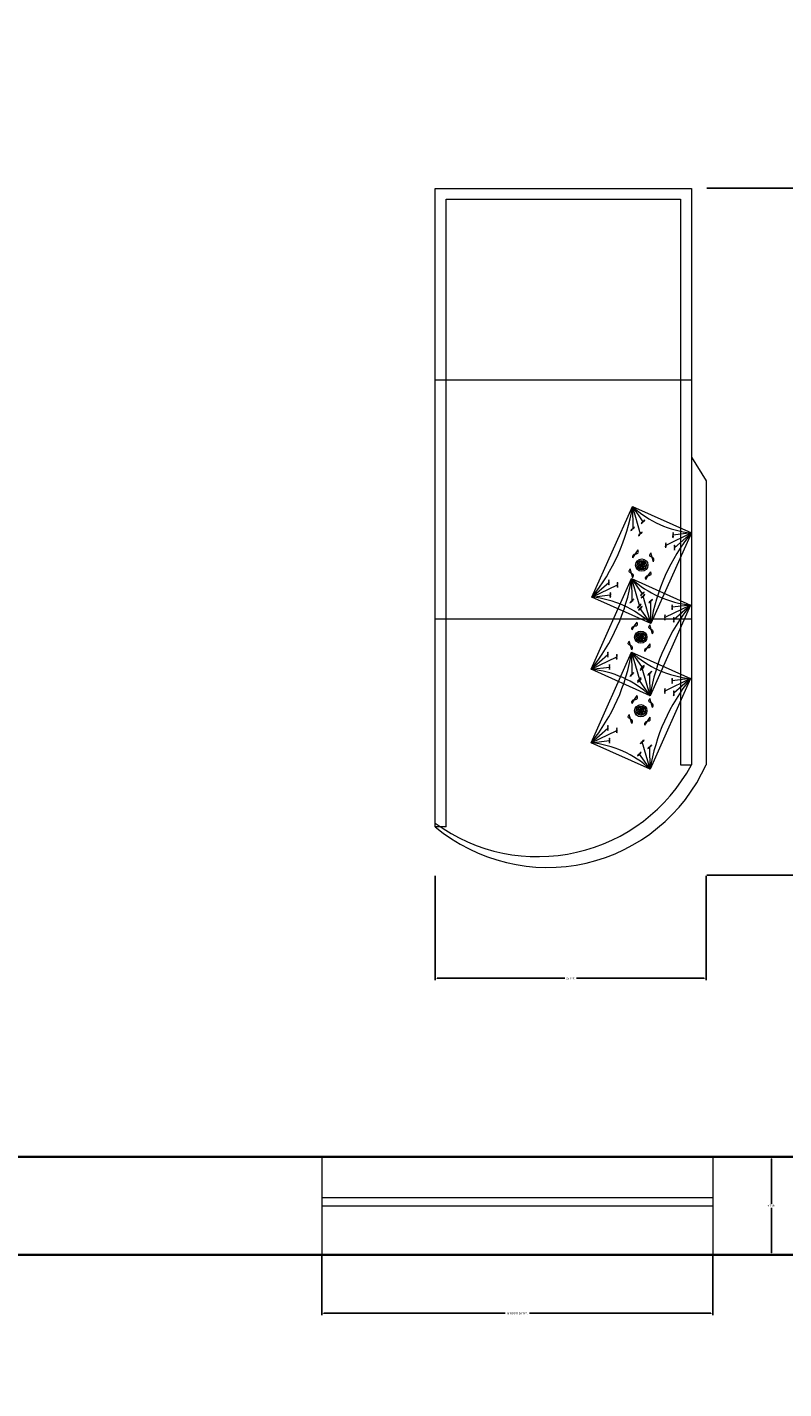
# Model space of a CAD drawing. Units: inches. Extents: x -61 to 1599, y -1316 to 257.
# Tile 189 of 204: x 1163 to 1233, y -454 to -328. Entities that reach past the tile are written whole.
import ezdxf

# ---------------------------------------------------------------- set-up
doc = ezdxf.new("R2010")
doc.units = ezdxf.units.IN
doc.header["$MEASUREMENT"] = 0
for name, color, linetype, lineweight in [('A-ANNO-DIMS', 2, 'Continuous', 18), ('FURNITURE', 83, 'Continuous', 18), ('WALLS', 4, 'Continuous', 35), ('WINDOWS', 220, 'Continuous', 18)]:
    doc.layers.add(name, color=color, linetype=linetype, lineweight=lineweight)
doc.styles.get("Standard").update_dxf_attribs({"font": 'arial.ttf'})
doc.dimstyles.get("Standard").update_dxf_attribs({"dimtxt": 0.18, "dimasz": 0.18, "dimexe": 0.18, "dimexo": 0.0625, "dimgap": 0.09, "dimtad": 0, "dimtih": 1, "dimtoh": 1, "dimdec": 0, "dimzin": 0, "dimdsep": 46, "dimlunit": 3, "dimtxsty": 'Standard', "dimcen": 0.09, "dimadec": 0, "dimazin": 0, "dimtfac": 1, "dimtdec": 0, "dimtofl": 0, "dimtmove": 0, "dimatfit": 3, "dimfxl": 1, "dimtolj": 1, "dimtzin": 0, "dimarcsym": 0})

# ---------------------------------------------------------------- blocks, each defined once
blk = doc.blocks.new('WIN-36IN-2')
for p, q in [((0, 9), (0, 0)), ((36, 9), (36, 0)), ((0, 5.26), (36, 5.26)), ((0, 4.5), (36, 4.5)), ((0, 4.5), (36, 4.5))]:
    blk.add_line(p, q)
blk = doc.blocks.new('MASTER-BEDROOM-CONSOLE')
for p, q in [((0, 44.89), (23.59, 44.89)), ((23.59, 37.78), (23.59, 9.44)), ((23.59, 37.78), (24.94, 35.59)), ((24.94, 35.59), (24.94, 9.46)), ((18.16, 33.23), (18.88, 30.7)), ((18.16, 33.23), (19.13, 31.83)), ((18.16, 33.23), (18.18, 31.17)), ((23.59, 30.8), (21.23, 29.65)), ((23.59, 30.8), (21.89, 30.59)), ((23.59, 30.8), (22.04, 29.44)), ((18.2, 28.51), (18.44, 28.87)), ((18.44, 28.87), (18.68, 29.23)), ((19.96, 28.55), (19.84, 28.97)), ((19.01, 27.84), (18.62, 28.02)), ((19.01, 27.84), (18.71, 27.53)), ((19.01, 27.84), (18.83, 27.45)), ((19.01, 27.84), (18.89, 28.25)), ((19.18, 28.23), (19.01, 27.84)), ((19.31, 28.15), (19.01, 27.84)), ((19.4, 27.66), (19.01, 27.84)), ((19.13, 27.43), (19.01, 27.84)), ((20.09, 28.14), (19.96, 28.55)), ((18.06, 27.07), (17.94, 27.48)), ((18.18, 26.66), (18.06, 27.07)), ((18.08, 26.59), (18.8, 24.06)), ((18.08, 26.59), (19.06, 25.19)), ((18.08, 26.59), (18.1, 24.53)), ((19.38, 26.52), (19.62, 26.88)), ((19.62, 26.88), (19.86, 27.23)), ((14.43, 24.88), (15.98, 26.24)), ((14.43, 24.88), (16.79, 26.03)), ((14.43, 24.88), (16.12, 25.09)), ((19.85, 22.45), (18.88, 23.85)), ((19.85, 22.45), (19.14, 24.98)), ((19.85, 22.45), (19.84, 24.51)), ((23.51, 24.16), (21.15, 23.01)), ((23.51, 24.16), (21.82, 23.95)), ((23.51, 24.16), (21.96, 22.8)), ((0, 22.89), (23.59, 22.89)), ((18.36, 22.23), (18.6, 22.59)), ((18.12, 21.87), (18.36, 22.23)), ((18.93, 21.2), (18.54, 21.38)), ((18.93, 21.2), (18.81, 21.61)), ((19.11, 21.59), (18.93, 21.2)), ((19.23, 21.51), (18.93, 21.2)), ((19.89, 21.91), (19.76, 22.33)), ((20.01, 21.5), (19.89, 21.91)), ((17.98, 20.43), (17.86, 20.84)), ((18.11, 20.02), (17.98, 20.43)), ((18.93, 21.2), (18.63, 20.89)), ((18.93, 21.2), (18.75, 20.81)), ((19.32, 21.02), (18.93, 21.2)), ((19.05, 20.79), (18.93, 21.2)), ((19.3, 19.88), (19.54, 20.24)), ((19.54, 20.24), (19.78, 20.59)), ((14.35, 18.24), (15.9, 19.6)), ((14.35, 18.24), (16.71, 19.39)), ((18.08, 19.82), (18.8, 17.29)), ((18.08, 19.82), (19.06, 18.42)), ((18.08, 19.82), (18.1, 17.76)), ((14.35, 18.24), (16.04, 18.45)), ((19.78, 15.81), (19.06, 18.34)), ((19.78, 15.81), (19.76, 17.87)), ((19.78, 15.81), (18.8, 17.21)), ((23.51, 17.39), (21.15, 16.24)), ((23.51, 17.39), (21.82, 17.18)), ((23.51, 17.39), (21.96, 16.03)), ((18.12, 15.1), (18.36, 15.46)), ((18.36, 15.46), (18.6, 15.82)), ((19.89, 15.14), (19.76, 15.56)), ((20.01, 14.73), (19.89, 15.14)), ((17.98, 13.66), (17.86, 14.08)), ((18.93, 14.43), (18.54, 14.61)), ((18.93, 14.43), (18.63, 14.12)), ((18.93, 14.43), (18.75, 14.04)), ((18.93, 14.43), (18.81, 14.84)), ((19.11, 14.82), (18.93, 14.43)), ((19.23, 14.74), (18.93, 14.43)), ((19.32, 14.26), (18.93, 14.43)), ((19.05, 14.02), (18.93, 14.43)), ((19.54, 13.47), (19.78, 13.83)), ((14.35, 11.47), (15.9, 12.83)), ((14.35, 11.47), (16.71, 12.62)), ((18.11, 13.25), (17.98, 13.66)), ((19.3, 13.11), (19.54, 13.47)), ((14.35, 11.47), (16.04, 11.68)), ((19.78, 9.04), (19.06, 11.57)), ((19.78, 9.04), (18.8, 10.44)), ((19.78, 9.04), (19.76, 11.1)), ((22.59, 9.44), (23.59, 9.44)), ((1, 3.75), (0, 3.75))]:
    blk.add_line(p, q)
for points in [[(0, 3.75), (0, 62.52), (23.59, 62.52), (23.59, 9.44)], [(1, 3.75), (1, 61.52), (22.59, 61.52), (22.59, 9.44)]]:
    blk.add_lwpolyline(points)
for points in [[(14.43, 24.88), (18.16, 33.23), (23.59, 30.8), (19.85, 22.45)], [(14.35, 18.24), (18.08, 26.59), (23.51, 24.16), (19.78, 15.81)], [(14.35, 11.47), (18.08, 19.82), (23.51, 17.39), (19.78, 9.04)]]:
    blk.add_lwpolyline(points, close=True)
for centre, radius in [((19.01, 27.84), 0.567), ((19.01, 27.84), 0.567), ((19.01, 27.84), 0.43), ((18.93, 21.2), 0.567), ((18.93, 21.2), 0.567), ((18.93, 21.2), 0.43), ((18.93, 14.43), 0.567), ((18.93, 14.43), 0.567), ((18.93, 14.43), 0.43)]:
    blk.add_circle(centre, radius)
for centre, radius, start, end in [((0.46, 36.13), 17.94, 321.1446, 350.6879), ((24.49, 40.12), 9.36, 227.4013, 264.4312), ((19.17, 31.62), 0.209, 99.3213, 167.2974), ((18.92, 31.88), 0.214, 280.2125, 346.4062), ((19.1, 32.04), 0.214, 280.2125, 346.4062), ((19.34, 31.78), 0.209, 99.3213, 167.2974), ((18.22, 30.96), 0.209, 99.3213, 167.2974), ((17.97, 31.22), 0.214, 280.2125, 346.4062), ((18.14, 31.38), 0.214, 280.2125, 346.4062), ((18.39, 31.12), 0.209, 99.3213, 167.2974), ((18.91, 30.5), 0.209, 99.3213, 167.2974), ((18.67, 30.75), 0.214, 280.2125, 346.4062), ((18.84, 30.92), 0.214, 280.2125, 346.4062), ((19.08, 30.66), 0.209, 99.3213, 167.2974), ((37.56, 19.55), 17.94, 141.1446, 170.6879), ((22.08, 30.7), 0.214, 145.4264, 211.62), ((22.07, 30.47), 0.214, 145.4264, 211.62), ((21.72, 30.71), 0.209, 324.5352, 32.5112), ((21.72, 30.48), 0.209, 324.5352, 32.5112), ((21.4, 29.53), 0.214, 145.4264, 211.62), ((21.41, 29.77), 0.214, 145.4264, 211.62), ((21.05, 29.54), 0.209, 324.5352, 32.5112), ((21.06, 29.78), 0.209, 324.5352, 32.5112), ((22.21, 29.32), 0.214, 145.4264, 211.62), ((22.22, 29.56), 0.214, 145.4264, 211.62), ((21.86, 29.33), 0.209, 324.5352, 32.5112), ((21.87, 29.56), 0.209, 324.5352, 32.5112), ((0.38, 29.49), 17.94, 321.1446, 350.6879), ((16.15, 26.35), 0.209, 144.5352, 212.5112), ((15.8, 26.36), 0.214, 325.4264, 31.62), ((24.42, 33.48), 9.36, 227.4013, 264.4312), ((16.15, 26.12), 0.209, 144.5352, 212.5112), ((15.8, 26.13), 0.214, 325.4264, 31.62), ((16.29, 24.97), 0.209, 144.5352, 212.5112), ((16.3, 25.2), 0.209, 144.5352, 212.5112), ((15.95, 25.21), 0.214, 325.4264, 31.62), ((15.94, 24.98), 0.214, 325.4264, 31.62), ((16.96, 25.9), 0.209, 144.5352, 212.5112), ((16.96, 26.14), 0.209, 144.5352, 212.5112), ((16.61, 25.91), 0.214, 325.4264, 31.62), ((16.61, 26.15), 0.214, 325.4264, 31.62), ((19.09, 24.98), 0.209, 99.3213, 167.2974), ((18.85, 25.24), 0.214, 280.2125, 346.4062), ((19.02, 25.4), 0.214, 280.2125, 346.4062), ((19.26, 25.14), 0.209, 99.3213, 167.2974), ((19.1, 25.18), 0.209, 279.3213, 347.2974), ((19.35, 24.93), 0.214, 100.2125, 166.4062), ((13.52, 15.57), 9.36, 47.4013, 84.4312), ((18.14, 24.32), 0.209, 99.3213, 167.2974), ((17.89, 24.58), 0.214, 280.2125, 346.4062), ((18.06, 24.74), 0.214, 280.2125, 346.4062), ((18.31, 24.48), 0.209, 99.3213, 167.2974), ((18.83, 23.86), 0.209, 99.3213, 167.2974), ((18.59, 24.11), 0.214, 280.2125, 346.4062), ((18.92, 23.64), 0.214, 100.2125, 166.4062), ((18.68, 23.9), 0.209, 279.3213, 347.2974), ((18.76, 24.28), 0.214, 280.2125, 346.4062), ((19, 24.02), 0.209, 99.3213, 167.2974), ((18.85, 24.06), 0.209, 279.3213, 347.2974), ((19.09, 23.8), 0.214, 100.2125, 166.4062), ((19.18, 24.77), 0.214, 100.2125, 166.4062), ((18.93, 25.02), 0.209, 279.3213, 347.2974), ((19.87, 24.3), 0.214, 100.2125, 166.4062), ((19.63, 24.56), 0.209, 279.3213, 347.2974), ((37.48, 12.91), 17.94, 141.1446, 170.6879), ((19.8, 24.72), 0.209, 279.3213, 347.2974), ((20.04, 24.46), 0.214, 100.2125, 166.4062), ((22, 24.06), 0.214, 145.4264, 211.62), ((21.99, 23.83), 0.214, 145.4264, 211.62), ((21.64, 23.84), 0.209, 324.5352, 32.5112), ((21.65, 24.07), 0.209, 324.5352, 32.5112), ((21.33, 22.89), 0.214, 145.4264, 211.62), ((21.33, 23.13), 0.214, 145.4264, 211.62), ((20.97, 22.9), 0.209, 324.5352, 32.5112), ((20.98, 23.14), 0.209, 324.5352, 32.5112), ((22.14, 22.68), 0.214, 145.4264, 211.62), ((22.14, 22.92), 0.214, 145.4264, 211.62), ((21.78, 22.69), 0.209, 324.5352, 32.5112), ((21.79, 22.92), 0.209, 324.5352, 32.5112), ((0.38, 22.72), 17.94, 321.1446, 350.6879), ((16.07, 19.48), 0.209, 144.5352, 212.5112), ((16.08, 19.71), 0.209, 144.5352, 212.5112), ((15.72, 19.49), 0.214, 325.4264, 31.62), ((15.72, 19.72), 0.214, 325.4264, 31.62), ((16.88, 19.26), 0.209, 144.5352, 212.5112), ((16.89, 19.5), 0.209, 144.5352, 212.5112), ((16.53, 19.27), 0.214, 325.4264, 31.62), ((16.53, 19.51), 0.214, 325.4264, 31.62), ((24.42, 26.71), 9.36, 227.4013, 264.4312), ((13.44, 8.93), 9.36, 47.4013, 84.4312), ((16.21, 18.33), 0.209, 144.5352, 212.5112), ((16.22, 18.56), 0.209, 144.5352, 212.5112), ((15.87, 18.57), 0.214, 325.4264, 31.62), ((15.86, 18.34), 0.214, 325.4264, 31.62), ((18.14, 17.55), 0.209, 99.3213, 167.2974), ((17.89, 17.81), 0.214, 280.2125, 346.4062), ((18.06, 17.97), 0.214, 280.2125, 346.4062), ((18.31, 17.71), 0.209, 99.3213, 167.2974), ((19.09, 18.21), 0.209, 99.3213, 167.2974), ((18.85, 18.47), 0.214, 280.2125, 346.4062), ((19.1, 18.13), 0.214, 100.2125, 166.4062), ((18.85, 18.38), 0.209, 279.3213, 347.2974), ((19.02, 18.63), 0.214, 280.2125, 346.4062), ((19.26, 18.37), 0.209, 99.3213, 167.2974), ((19.03, 18.54), 0.209, 279.3213, 347.2974), ((19.27, 18.29), 0.214, 100.2125, 166.4062), ((19.79, 17.66), 0.214, 100.2125, 166.4062), ((19.55, 17.92), 0.209, 279.3213, 347.2974), ((19.72, 18.08), 0.209, 279.3213, 347.2974), ((19.97, 17.82), 0.214, 100.2125, 166.4062), ((18.83, 17.09), 0.209, 99.3213, 167.2974), ((18.59, 17.35), 0.214, 280.2125, 346.4062), ((18.84, 17), 0.214, 100.2125, 166.4062), ((18.6, 17.26), 0.209, 279.3213, 347.2974), ((18.76, 17.51), 0.214, 280.2125, 346.4062), ((19, 17.25), 0.209, 99.3213, 167.2974), ((18.77, 17.42), 0.209, 279.3213, 347.2974), ((19.01, 17.16), 0.214, 100.2125, 166.4062), ((37.48, 6.14), 17.94, 141.1446, 170.6879), ((21.33, 16.36), 0.214, 145.4264, 211.62), ((20.98, 16.37), 0.209, 324.5352, 32.5112), ((22, 17.3), 0.214, 145.4264, 211.62), ((21.99, 17.06), 0.214, 145.4264, 211.62), ((21.64, 17.07), 0.209, 324.5352, 32.5112), ((21.65, 17.3), 0.209, 324.5352, 32.5112), ((21.33, 16.12), 0.214, 145.4264, 211.62), ((20.97, 16.13), 0.209, 324.5352, 32.5112), ((22.14, 15.91), 0.214, 145.4264, 211.62), ((22.14, 16.15), 0.214, 145.4264, 211.62), ((21.78, 15.92), 0.209, 324.5352, 32.5112), ((21.79, 16.15), 0.209, 324.5352, 32.5112), ((16.07, 12.71), 0.209, 144.5352, 212.5112), ((16.08, 12.94), 0.209, 144.5352, 212.5112), ((15.72, 12.72), 0.214, 325.4264, 31.62), ((15.72, 12.95), 0.214, 325.4264, 31.62), ((16.88, 12.5), 0.209, 144.5352, 212.5112), ((16.89, 12.73), 0.209, 144.5352, 212.5112), ((16.53, 12.5), 0.214, 325.4264, 31.62), ((16.53, 12.74), 0.214, 325.4264, 31.62), ((13.44, 2.16), 9.36, 47.4013, 84.4312), ((16.21, 11.56), 0.209, 144.5352, 212.5112), ((16.22, 11.79), 0.209, 144.5352, 212.5112), ((15.87, 11.8), 0.214, 325.4264, 31.62), ((15.86, 11.57), 0.214, 325.4264, 31.62), ((19.1, 11.36), 0.214, 100.2125, 166.4062), ((18.85, 11.61), 0.209, 279.3213, 347.2974), ((19.03, 11.77), 0.209, 279.3213, 347.2974), ((19.27, 11.52), 0.214, 100.2125, 166.4062), ((18.84, 10.23), 0.214, 100.2125, 166.4062), ((18.6, 10.49), 0.209, 279.3213, 347.2974), ((18.77, 10.65), 0.209, 279.3213, 347.2974), ((19.01, 10.39), 0.214, 100.2125, 166.4062), ((19.79, 10.89), 0.214, 100.2125, 166.4062), ((19.55, 11.15), 0.209, 279.3213, 347.2974), ((19.72, 11.31), 0.209, 279.3213, 347.2974), ((19.97, 11.05), 0.214, 100.2125, 166.4062), ((10.31, 16.05), 16.05, 230.0449, 335.7344), ((9.45, 17.04), 16.05, 233.9382, 331.7264)]:
    blk.add_arc(centre, radius, start, end)
for points in [[(18.2, 28.51), (18.19, 28.6), (18.17, 28.79), (18.44, 28.88), (18.78, 28.9), (18.67, 29.16), (18.68, 29.23)], [(20.09, 28.14), (20.12, 28.23), (20.2, 28.4), (19.97, 28.57), (19.65, 28.68), (19.83, 28.9), (19.84, 28.97)], [(19.4, 27.66), (19.36, 27.75), (19.28, 27.92), (19, 27.85), (18.71, 27.68), (18.66, 27.96), (18.62, 28.02)], [(19.31, 28.15), (19.3, 28.05), (19.29, 27.87), (19.01, 27.83), (18.67, 27.88), (18.73, 27.6), (18.71, 27.53)], [(19.13, 27.43), (19.17, 27.51), (19.25, 27.69), (19.02, 27.85), (18.69, 27.97), (18.87, 28.18), (18.89, 28.25)], [(19.18, 28.23), (19.1, 28.19), (18.93, 28.11), (18.99, 27.83), (19.17, 27.54), (18.89, 27.49), (18.83, 27.45)], [(18.18, 26.66), (18.22, 26.75), (18.3, 26.92), (18.07, 27.09), (17.75, 27.2), (17.93, 27.41), (17.94, 27.48)], [(19.38, 26.52), (19.37, 26.61), (19.34, 26.8), (19.61, 26.89), (19.96, 26.9), (19.85, 27.16), (19.86, 27.23)], [(18.12, 21.87), (18.11, 21.96), (18.09, 22.15), (18.36, 22.24), (18.7, 22.26), (18.59, 22.52), (18.6, 22.59)], [(19.32, 21.02), (19.28, 21.11), (19.2, 21.28), (18.92, 21.21), (18.63, 21.04), (18.58, 21.32), (18.54, 21.38)], [(19.23, 21.51), (19.22, 21.41), (19.21, 21.23), (18.93, 21.19), (18.59, 21.24), (18.65, 20.96), (18.63, 20.89)], [(19.05, 20.79), (19.09, 20.87), (19.17, 21.05), (18.94, 21.21), (18.62, 21.33), (18.8, 21.54), (18.81, 21.61)], [(19.11, 21.59), (19.02, 21.55), (18.85, 21.47), (18.92, 21.19), (19.09, 20.9), (18.81, 20.85), (18.75, 20.81)], [(20.01, 21.5), (20.05, 21.59), (20.12, 21.76), (19.89, 21.93), (19.57, 22.04), (19.75, 22.26), (19.76, 22.33)], [(18.11, 20.02), (18.14, 20.11), (18.22, 20.28), (17.99, 20.45), (17.67, 20.56), (17.85, 20.77), (17.86, 20.84)], [(19.3, 19.88), (19.29, 19.97), (19.27, 20.16), (19.54, 20.25), (19.88, 20.26), (19.77, 20.52), (19.78, 20.59)], [(18.12, 15.1), (18.11, 15.19), (18.09, 15.38), (18.36, 15.47), (18.7, 15.49), (18.59, 15.75), (18.6, 15.82)], [(20.01, 14.73), (20.05, 14.82), (20.12, 14.99), (19.89, 15.16), (19.57, 15.27), (19.75, 15.49), (19.76, 15.56)], [(18.11, 13.25), (18.14, 13.34), (18.22, 13.51), (17.99, 13.68), (17.67, 13.79), (17.85, 14.01), (17.86, 14.08)], [(19.32, 14.26), (19.28, 14.34), (19.2, 14.51), (18.92, 14.44), (18.63, 14.27), (18.58, 14.55), (18.54, 14.61)], [(19.23, 14.74), (19.22, 14.64), (19.21, 14.46), (18.93, 14.42), (18.59, 14.47), (18.65, 14.19), (18.63, 14.12)], [(19.05, 14.02), (19.09, 14.1), (19.17, 14.28), (18.94, 14.44), (18.62, 14.56), (18.8, 14.77), (18.81, 14.84)], [(19.11, 14.82), (19.02, 14.78), (18.85, 14.7), (18.92, 14.43), (19.09, 14.13), (18.81, 14.08), (18.75, 14.04)], [(19.3, 13.11), (19.29, 13.2), (19.27, 13.39), (19.54, 13.48), (19.88, 13.49), (19.77, 13.75), (19.78, 13.83)]]:
    blk.add_open_spline(points, degree=3, knots=[0, 0, 0, 0, 0.249187, 0.498374, 0.766554, 1.034734, 1.034734, 1.034734, 1.034734])
blk = doc.blocks.new('*D640')
at = {"layer": 'A-ANNO-DIMS', "color": 0, "lineweight": -2, "transparency": 16777216}
for p, q in [((1190.16, -441.39), (1190.16, -446.9)), ((1226.16, -441.39), (1226.16, -446.9)), ((1190.34, -446.72), (1207.04, -446.72)), ((1225.98, -446.72), (1209.28, -446.72))]:
    blk.add_line(p, q, dxfattribs=at)
at = {"layer": 'A-ANNO-DIMS', "color": 0, "transparency": 16777216}
for points in [[(1190.34, -446.69), (1190.34, -446.75), (1190.16, -446.72)], [(1225.98, -446.69), (1225.98, -446.75), (1226.16, -446.72)]]:
    blk.add_solid(points, dxfattribs=at)
at = {"layer": 'DEFPOINTS', "color": 0, "transparency": 16777216}
for p in [(1190.16, -441.32), (1226.16, -441.32), (1226.16, -446.72)]:
    blk.add_point(p, dxfattribs=at)
at = {"layer": 'A-ANNO-DIMS', "color": 0, "transparency": 16777216, "insert": (1208.16, -446.72), "char_height": 0.18, "attachment_point": 5}
blk.add_mtext('\\A1;WINDOW 36 TYP.', dxfattribs=at)
blk = doc.blocks.new('*D641')
at = {"layer": 'A-ANNO-DIMS', "color": 0, "lineweight": -2, "transparency": 16777216}
for p, q in [((1226.22, -432.32), (1231.74, -432.32)), ((1231.56, -432.5), (1231.56, -436.64)), ((1231.56, -441.14), (1231.56, -437)), ((1226.22, -441.32), (1231.74, -441.32))]:
    blk.add_line(p, q, dxfattribs=at)
at = {"layer": 'A-ANNO-DIMS', "color": 0, "transparency": 16777216}
for points in [[(1231.53, -432.5), (1231.59, -432.5), (1231.56, -432.32)], [(1231.53, -441.14), (1231.59, -441.14), (1231.56, -441.32)]]:
    blk.add_solid(points, dxfattribs=at)
at = {"layer": 'DEFPOINTS', "color": 0, "transparency": 16777216}
for p in [(1226.16, -432.32), (1231.56, -432.32), (1226.16, -441.32)]:
    blk.add_point(p, dxfattribs=at)
at = {"layer": 'A-ANNO-DIMS', "color": 0, "transparency": 16777216, "insert": (1231.56, -436.82), "char_height": 0.18, "attachment_point": 5}
blk.add_mtext('\\A1;9 TYP.', dxfattribs=at)
blk = doc.blocks.new('*D664')
at = {"layer": 'A-ANNO-DIMS', "color": 0, "lineweight": -2, "transparency": 16777216}
for p, q in [((1225.61, -343.14), (1235.21, -343.14)), ((1235.03, -343.32), (1235.03, -374.58)), ((1235.03, -406.2), (1235.03, -374.95)), ((1225.61, -406.38), (1235.21, -406.38))]:
    blk.add_line(p, q, dxfattribs=at)
at = {"layer": 'A-ANNO-DIMS', "color": 0, "transparency": 16777216}
for points in [[(1235, -343.32), (1235.06, -343.32), (1235.03, -343.14)], [(1235, -406.2), (1235.06, -406.2), (1235.03, -406.38)]]:
    blk.add_solid(points, dxfattribs=at)
at = {"layer": 'DEFPOINTS', "color": 0, "transparency": 16777216}
for p in [(1225.55, -343.14), (1235.03, -343.14), (1225.55, -406.38)]:
    blk.add_point(p, dxfattribs=at)
at = {"layer": 'A-ANNO-DIMS', "color": 0, "transparency": 16777216, "insert": (1235.03, -374.76), "char_height": 0.18, "attachment_point": 5}
blk.add_mtext('\\A1;CONSOLE 63 TYP.', dxfattribs=at)
blk = doc.blocks.new('*D665')
at = {"layer": 'A-ANNO-DIMS', "color": 0, "lineweight": -2, "transparency": 16777216}
for p, q in [((1200.6, -406.45), (1200.6, -416.05)), ((1225.55, -406.45), (1225.55, -416.05)), ((1200.78, -415.87), (1212.54, -415.87)), ((1225.37, -415.87), (1213.6, -415.87))]:
    blk.add_line(p, q, dxfattribs=at)
at = {"layer": 'A-ANNO-DIMS', "color": 0, "transparency": 16777216}
for points in [[(1200.78, -415.84), (1200.78, -415.9), (1200.6, -415.87)], [(1225.37, -415.84), (1225.37, -415.9), (1225.55, -415.87)]]:
    blk.add_solid(points, dxfattribs=at)
at = {"layer": 'DEFPOINTS', "color": 0, "transparency": 16777216}
for p in [(1200.6, -406.38), (1225.55, -406.38), (1225.55, -415.87)]:
    blk.add_point(p, dxfattribs=at)
at = {"layer": 'A-ANNO-DIMS', "color": 0, "transparency": 16777216, "insert": (1213.07, -415.87), "char_height": 0.18, "attachment_point": 5}
blk.add_mtext('\\A1;25 TYP.', dxfattribs=at)
blk = doc.blocks.new('*D698')
at = {"layer": 'A-ANNO-DIMS', "color": 0, "lineweight": -2, "transparency": 16777216}
for p, q in [((644.77, -167.17), (1598.48, -167.17)), ((1598.3, -167.35), (1598.3, -363.99)), ((1598.3, -560.99), (1598.3, -364.35)), ((644.77, -561.17), (1598.48, -561.17))]:
    blk.add_line(p, q, dxfattribs=at)
at = {"layer": 'A-ANNO-DIMS', "color": 0, "transparency": 16777216}
for points in [[(1598.27, -167.35), (1598.33, -167.35), (1598.3, -167.17)], [(1598.27, -560.99), (1598.33, -560.99), (1598.3, -561.17)]]:
    blk.add_solid(points, dxfattribs=at)
at = {"layer": 'DEFPOINTS', "color": 0, "transparency": 16777216}
for p in [(644.7, -167.17), (1598.3, -167.17), (644.7, -561.17)]:
    blk.add_point(p, dxfattribs=at)
at = {"layer": 'A-ANNO-DIMS', "color": 0, "transparency": 16777216, "insert": (1598.3, -364.17), "char_height": 0.18, "attachment_point": 5}
blk.add_mtext('\\A1;394', dxfattribs=at)

msp = doc.modelspace()

# ---------------------------------------------------------------- linework, layer by layer
at = {"layer": 'WALLS'}
for p, q in [((1065.7028, -432.3229), (1215.7028, -432.3229)), ((1215.7028, -432.3229), (1237.7028, -432.3229)), ((992.7028, -441.3229), (1215.7028, -441.3229)), ((1215.7028, -441.3229), (1297.7028, -441.3229))]:
    msp.add_line(p, q, dxfattribs=at)

# ---------------------------------------------------------------- block references
at = {"layer": 'FURNITURE'}
msp.add_blockref('MASTER-BEDROOM-CONSOLE', (1200.602, -405.667), dxfattribs=at)
at = {"layer": 'WINDOWS'}
msp.add_blockref('WIN-36IN-2', (1190.158, -441.323), dxfattribs=at)

# ---------------------------------------------------------------- dimensions: what is measured, and where the dimension line sits
at = {"layer": 'A-ANNO-DIMS'}
dim = msp.add_linear_dim(base=(1598.3028, -167.169), p1=(644.7028, -561.169), p2=(644.7028, -167.169), angle=90, dimstyle='Standard', override={"dimdec": 0, "dimlfac": 1, "dimrnd": 0, "dimzin": 0, "dimdsep": 46, "dimlunit": 2}, dxfattribs=at)
dim.commit()
dim.dimension.update_dxf_attribs({"geometry": '*D698', "text_midpoint": (1598.3028, -364.169)})
for base, p1, p2, text, picture, middle in [((1235.0311, -343.1432), (1225.5451, -406.3834), (1225.5451, -343.1432), 'CONSOLE <> TYP.', '*D664', (1235.0311, -374.7633)), ((1231.5584, -432.3229), (1226.1584, -441.3229), (1226.1584, -432.3229), '<> TYP.', '*D641', (1231.5584, -436.8229))]:
    dim = msp.add_linear_dim(base=base, p1=p1, p2=p2, angle=90, text=text, dimstyle='Standard', override={"dimdec": 0, "dimlfac": 1, "dimrnd": 0, "dimzin": 0, "dimdsep": 46, "dimlunit": 2}, dxfattribs=at)
    dim.commit()
    dim.dimension.update_dxf_attribs({"geometry": picture, "text_midpoint": middle})
for base, p1, p2, text, picture, middle in [((1225.5451, -415.8694), (1200.6016, -406.3834), (1225.5451, -406.3834), '<> TYP.', '*D665', (1213.0733, -415.8694)), ((1226.1584, -446.7229), (1190.1584, -441.3229), (1226.1584, -441.3229), 'WINDOW <> TYP.', '*D640', (1208.1584, -446.7229))]:
    dim = msp.add_linear_dim(base=base, p1=p1, p2=p2, text=text, dimstyle='Standard', override={"dimdec": 0, "dimlfac": 1, "dimrnd": 0, "dimzin": 0, "dimdsep": 46, "dimlunit": 2}, dxfattribs=at)
    dim.commit()
    dim.dimension.update_dxf_attribs({"geometry": picture, "text_midpoint": middle})

doc.saveas('drawing.dxf')
